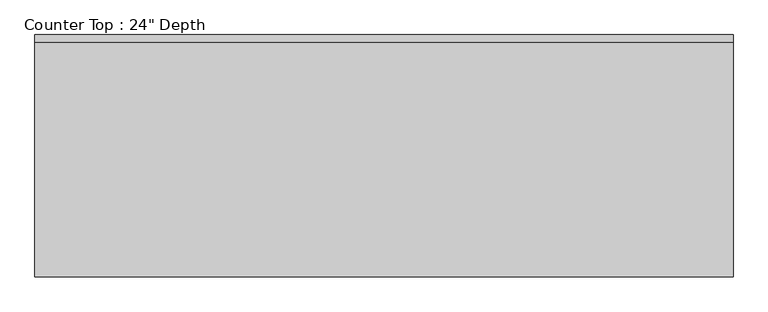
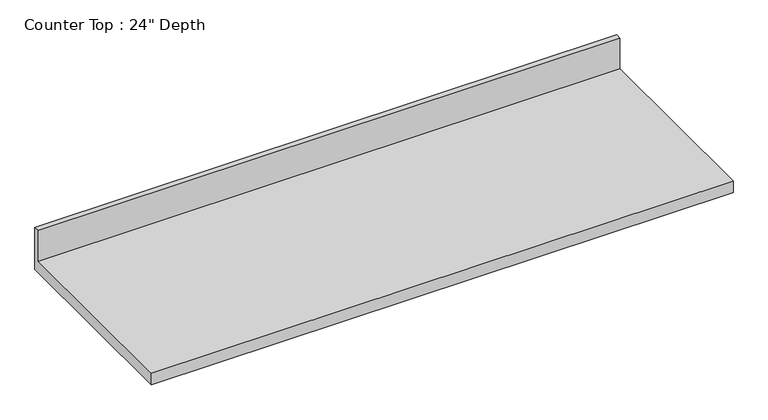
"""IFC4 building model written with IfcOpenShell, lengths in millimetres: furniture geometry."""

from ifc_helpers import new_model, si_unit, frame, origin, place, context, project, spatial, polyline, outline, extrude, source, transform, mapped, element, save


def furniture_6990e744(model_context):
    return source(origin(), model_context, "Body", "SweptSolid", [
        extrude(outline(polyline([(0.0, 1016.0), (0.0, 876.3), (-635.0, 876.3), (-635.0, 914.4), (-19.05, 914.4), (-19.05, 1016.0), (0.0, 1016.0)])), frame((-1200.4622951, 0.0, 0.0), z_axis=(1.0, 0.0, 0.0), x_axis=(0.0, 1.0, 0.0)), (0.0, 0.0, 1.0), 1828.8),
    ])


if __name__ == "__main__":
    model = new_model("IFC4")
    model_context = context("Model", 3, world=origin())
    ifc_project = project(units=[si_unit("LENGTHUNIT", "METRE", prefix="MILLI")], contexts=[model_context])
    site = spatial("IfcSite", under=ifc_project)
    building = spatial("IfcBuilding", under=site)
    placement = place(None, origin())
    furniture_shape = furniture_6990e744(model_context)
    element("IfcFurniture", 1, ObjectType="Counter Top : 24\" Depth", at=placement, inside=building, context=model_context, shape_type="MappedRepresentation", body=[
        mapped(furniture_shape, transform((0.0, 0.0, 0.0), x_axis=(1.0, 0.0, 0.0), y_axis=(0.0, 1.0, 0.0), z_axis=(0.0, 0.0, 1.0))),
    ])
    save(model, "model.ifc")

# Revit data of these elements
# Type "Counter Top : 24\" Depth"
#   Assembly Code = "C1030400"
#   Counter Thickness = 0' - 1 1/2"
#   Depth = 2' - 1"
#   Height = 3' - 0"
#   Length [instance default] = 8' - 0"
#   Counter Top Material = none
#   Default Elevation = 0
# Element 1 (IfcFurniture, "Counter Top : 24\" Depth")
#   Length = 6' - 0"
#   Materials on its faces: "Counter Top"
# Materials
#   "Counter Top": class "Wood", colour RGB 226 177 128, transparency 0
